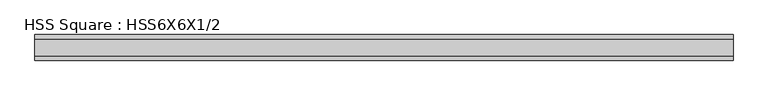
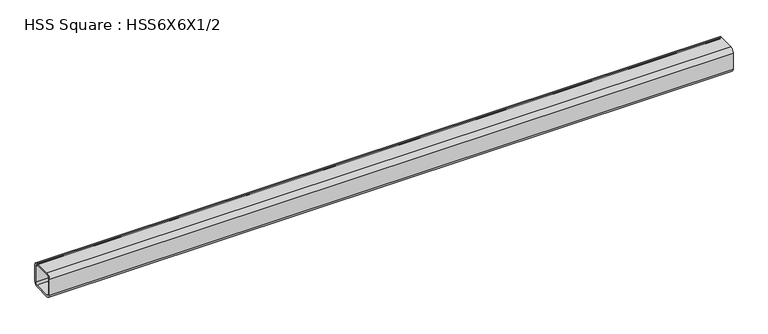
"""IFC4 building model written with IfcOpenShell, lengths in millimetres: member geometry, HSS Square : HSS6X6X1/2."""

from ifc_helpers import new_model, si_unit, point, frame, frame_2d, origin, place, context, project, spatial, polyline, circle_curve, trimmed, segment, composite_curve, outline, extrude, source, transform, mapped, element, save


def hss_square_hss6x6x1_2_e6555cf9(model_context):
    return source(origin(), model_context, "Body", "SweptSolid", [
        extrude(outline(composite_curve([segment(polyline([(76.2, 50.8), (76.2, -50.8)]), True, "CONTINUOUS"), segment(trimmed(circle_curve(frame_2d((50.8, -50.8)), 25.4), [point((76.2, -50.8))], [point((50.8, -76.2))], False, "CARTESIAN"), True, "CONTINUOUS"), segment(polyline([(50.8, -76.2), (-50.8, -76.2)]), True, "CONTINUOUS"), segment(trimmed(circle_curve(frame_2d((-50.8, -50.8)), 25.4), [point((-50.8, -76.2))], [point((-76.2, -50.8))], False, "CARTESIAN"), True, "CONTINUOUS"), segment(polyline([(-76.2, -50.8), (-76.2, 50.8)]), True, "CONTINUOUS"), segment(trimmed(circle_curve(frame_2d((-50.8, 50.8)), 25.4), [point((-76.2, 50.8))], [point((-50.8, 76.2))], False, "CARTESIAN"), True, "CONTINUOUS"), segment(polyline([(-50.8, 76.2), (50.8, 76.2)]), True, "CONTINUOUS"), segment(trimmed(circle_curve(frame_2d((50.8, 50.8)), 25.4), [point((50.8, 76.2))], [point((76.2, 50.8))], False, "CARTESIAN"), True, "CONTINUOUS")], self_intersect=False), holes=[composite_curve([segment(trimmed(circle_curve(frame_2d((-50.8, 50.8)), 12.7), [point((-50.8, 63.5))], [point((-63.5, 50.8))], True, "CARTESIAN"), True, "CONTINUOUS"), segment(polyline([(-63.5, 50.8), (-63.5, -50.8)]), True, "CONTINUOUS"), segment(trimmed(circle_curve(frame_2d((-50.8, -50.8)), 12.7), [point((-63.5, -50.8))], [point((-50.8, -63.5))], True, "CARTESIAN"), True, "CONTINUOUS"), segment(polyline([(-50.8, -63.5), (50.8, -63.5)]), True, "CONTINUOUS"), segment(trimmed(circle_curve(frame_2d((50.8, -50.8)), 12.7), [point((50.8, -63.5))], [point((63.5, -50.8))], True, "CARTESIAN"), True, "CONTINUOUS"), segment(polyline([(63.5, -50.8), (63.5, 50.8)]), True, "CONTINUOUS"), segment(trimmed(circle_curve(frame_2d((50.8, 50.8)), 12.7), [point((63.5, 50.8))], [point((50.8, 63.5))], True, "CARTESIAN"), True, "CONTINUOUS"), segment(polyline([(50.8, 63.5), (-50.8, 63.5)]), True, "CONTINUOUS")], self_intersect=False)]), frame((-2183.0973968, 0.0, 0.0), z_axis=(1.0, 0.0, 0.0), x_axis=(0.0, 1.0, 0.0)), (0.0, 0.0, 1.0), 4148.9536814),
    ])


if __name__ == "__main__":
    model = new_model("IFC4")
    model_context = context("Model", 3, world=origin())
    ifc_project = project(units=[si_unit("LENGTHUNIT", "METRE", prefix="MILLI")], contexts=[model_context])
    site = spatial("IfcSite", under=ifc_project)
    building = spatial("IfcBuilding", under=site)
    placement = place(None, origin())
    hss_square_hss6x6x1_2_shape = hss_square_hss6x6x1_2_e6555cf9(model_context)
    element("IfcMember", 1, ObjectType="HSS Square : HSS6X6X1/2", at=placement, inside=building, context=model_context, shape_type="MappedRepresentation", body=[
        mapped(hss_square_hss6x6x1_2_shape, transform((0.0, 0.0, 0.0), x_axis=(1.0, 0.0, 0.0), y_axis=(0.0, 1.0, 0.0), z_axis=(0.0, 0.0, 1.0))),
    ])
    save(model, "model.ifc")

# Revit data of these elements
# Type "HSS Square : HSS6X6X1/2"
#   Section Name Key = "HSS 6X6X1/2"
#   Assembly Code = "B10"
#   Width = 6.000"
#   Wall Nominal Thickness = 0.500"
#   Wall Design Thickness = 0.465"
#   Torsional Moment of Inertia = 81.10 in⁴
#   Torsional Modulus = 28.10 in³
#   Section Area = 9.74 in²
#   Plastic Modulus weak axis = 19.80 in³
#   Plastic Modulus strong axis = 19.80 in³
#   Outer Fillet = 1.000"
#   Nominal Weight = 35.24 lbf/ft
#   Moment of Inertia weak axis = 48.30 in⁴
#   Moment of Inertia strong axis = 48.30 in⁴
#   Inner Fillet = 0.500"
#   Height = 6.000"
#   Elastic Modulus weak axis = 16.10 in³
#   Elastic Modulus strong axis = 16.10 in³
#   Centroid Vertical = 3.000"
#   Centroid Horizontal = 3.000"
#   Length [instance default] = 5' - 0"
#   Structural Material [instance default] = Steel ASTM A500, Grade B, Rectangular and Square
#   Principal Axes Angle = 0
# Element 1 (IfcMember, "HSS Square : HSS6X6X1/2")
#   Structural Material = Steel ASTM A992
#   Materials on its faces: "Steel ASTM A992"
# Materials
#   "Steel ASTM A500, Grade B, Rectangular and Square": class "Metal", colour RGB 199 199 199, transparency 0, Description = "Carbon steel", Cost = 0
#   "Steel ASTM A992": class "Metal", colour RGB 199 199 199, transparency 0, Description = "Structural steel 50ksi", Cost = 0
